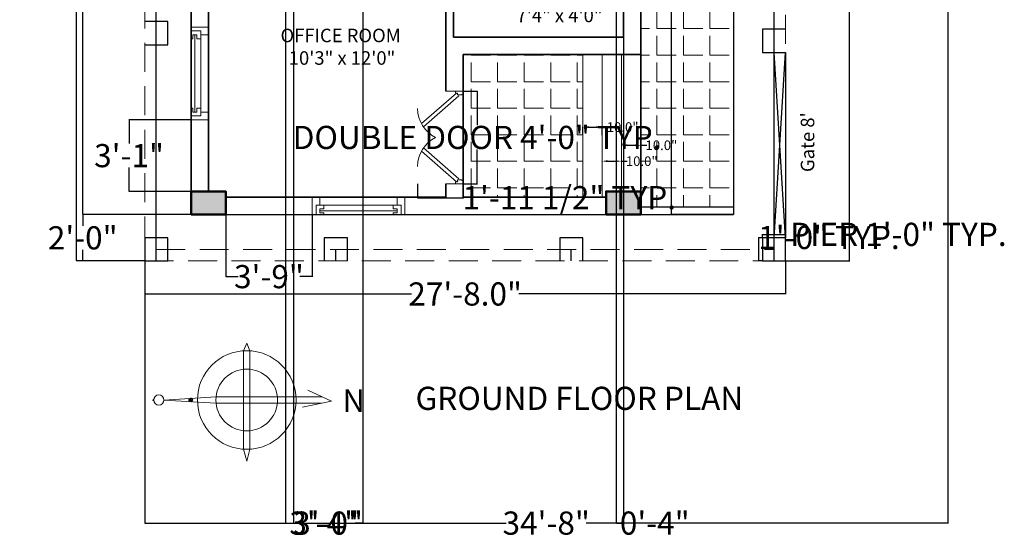
# Model space of a CAD drawing. Units: inches. Extents: x 1063 to 2718, y 423 to 1923.
# Tile 1 of 7: x 1086 to 1596, y 423 to 692. Entities that reach past the tile are written whole.
import ezdxf

# ---------------------------------------------------------------- set-up
doc = ezdxf.new("R2010")
doc.units = ezdxf.units.IN
doc.header["$LTSCALE"] = 6
doc.header["$MEASUREMENT"] = 0
doc.linetypes.add('HIDDEN', pattern=[0.375, 0.25, -0.125])
for name, color, linetype, lineweight in [('A-ANNO-DIMS', 2, 'Continuous', 18), ('A-ANNO-SYMB', 4, 'Continuous', 18), ('A-ANNO-TEXT', 7, 'Continuous', 18), ('A-ANNO-TITL', 7, 'Continuous', 35), ('A-AREA-IDEN', 7, 'Continuous', 18), ('A-COLS', 7, 'Continuous', 50), ('A-COLS-PATT', 252, 'Continuous', 13), ('A-DOOR', 2, 'Continuous', 18), ('A-FLOR', 7, 'Continuous', 25), ('A-FLOR-PATT', 9, 'Continuous', 13), ('A-FLOR-STRS', 7, 'Continuous', 18), ('A-GLAZ', 4, 'Continuous', 18), ('A-WALL', 7, 'Continuous', 35), ('C-GATE', 7, 'Continuous', 25), ('C-PROP', 7, 'Continuous', 25), ('C-PROP-HIDN', 7, 'HIDDEN', 18)]:
    doc.layers.add(name, color=color, linetype=linetype, lineweight=lineweight)
doc.styles.get("Standard").update_dxf_attribs({"font": 'arial.ttf'})
doc.dimstyles.get("Standard").update_dxf_attribs({"dimtxt": 12, "dimasz": 0.18, "dimexe": 0.18, "dimexo": 0.0625, "dimgap": 0.09, "dimtad": 0, "dimtih": 1, "dimtoh": 1, "dimdec": 1, "dimzin": 0, "dimdsep": 46, "dimlunit": 3, "dimtxsty": 'Standard', "dimcen": 0.09, "dimadec": 0, "dimazin": 0, "dimtfac": 1, "dimtdec": 1, "dimtofl": 0, "dimtmove": 0, "dimatfit": 3, "dimfxl": 1, "dimtolj": 1, "dimtzin": 0, "dimarcsym": 0})

# ---------------------------------------------------------------- blocks, each defined once
blk = doc.blocks.new('*D1')
at = {"layer": 'A-ANNO-DIMS', "color": 0, "lineweight": -2, "ltscale": 6, "transparency": 16777216}
for p, q in [((1150.86, 1085.12), (1115.44, 1085.12)), ((1115.62, 1084.94), (1115.62, 832.34)), ((1115.62, 567.3), (1115.62, 819.9)), ((1150.86, 567.12), (1115.44, 567.12))]:
    blk.add_line(p, q, dxfattribs=at)
at = {"layer": 'A-ANNO-DIMS', "color": 0, "ltscale": 6, "transparency": 16777216}
for points in [[(1115.59, 1084.94), (1115.65, 1084.94), (1115.62, 1085.12)], [(1115.59, 567.3), (1115.65, 567.3), (1115.62, 567.12)]]:
    blk.add_solid(points, dxfattribs=at)
at = {"layer": 'Defpoints', "color": 0, "ltscale": 6, "transparency": 16777216}
for p in [(1115.62, 1085.12), (1150.93, 1085.12), (1150.93, 567.12)]:
    blk.add_point(p, dxfattribs=at)
at = {"layer": 'A-ANNO-DIMS', "color": 0, "ltscale": 6, "transparency": 16777216, "insert": (1115.62, 826.12), "char_height": 12, "attachment_point": 5}
blk.add_mtext('\\A1;43\'-2.0"', dxfattribs=at)
blk = doc.blocks.new('*D2')
at = {"layer": 'A-ANNO-DIMS', "color": 0, "lineweight": -2, "ltscale": 6, "transparency": 16777216}
for p, q in [((1150.93, 567.06), (1150.93, 549.86)), ((1482.93, 567.06), (1482.93, 549.86)), ((1151.11, 550.04), (1289.13, 550.04)), ((1482.75, 550.04), (1344.72, 550.04))]:
    blk.add_line(p, q, dxfattribs=at)
at = {"layer": 'A-ANNO-DIMS', "color": 0, "ltscale": 6, "transparency": 16777216}
for points in [[(1151.11, 550.07), (1151.11, 550.01), (1150.93, 550.04)], [(1482.75, 550.07), (1482.75, 550.01), (1482.93, 550.04)]]:
    blk.add_solid(points, dxfattribs=at)
at = {"layer": 'Defpoints', "color": 0, "ltscale": 6, "transparency": 16777216}
for p in [(1150.93, 567.12), (1482.93, 567.12), (1482.93, 550.04)]:
    blk.add_point(p, dxfattribs=at)
at = {"layer": 'A-ANNO-DIMS', "color": 0, "ltscale": 6, "transparency": 16777216, "insert": (1316.93, 550.04), "char_height": 12, "attachment_point": 5}
blk.add_mtext('\\A1;27\'-8.0"', dxfattribs=at)
blk = doc.blocks.new('*D3')
at = {"layer": 'A-ANNO-DIMS', "color": 0, "lineweight": -2, "ltscale": 6, "transparency": 16777216}
for p, q in [((1482.99, 951.12), (1516.18, 951.12)), ((1516, 950.94), (1516, 765.34)), ((1516, 567.3), (1516, 752.9)), ((1482.99, 567.12), (1516.18, 567.12))]:
    blk.add_line(p, q, dxfattribs=at)
at = {"layer": 'A-ANNO-DIMS', "color": 0, "ltscale": 6, "transparency": 16777216}
for points in [[(1515.97, 950.94), (1516.03, 950.94), (1516, 951.12)], [(1515.97, 567.3), (1516.03, 567.3), (1516, 567.12)]]:
    blk.add_solid(points, dxfattribs=at)
at = {"layer": 'Defpoints', "color": 0, "ltscale": 6, "transparency": 16777216}
for p in [(1482.93, 951.12), (1516, 951.12), (1482.93, 567.12)]:
    blk.add_point(p, dxfattribs=at)
at = {"layer": 'A-ANNO-DIMS', "color": 0, "ltscale": 6, "transparency": 16777216, "insert": (1516, 759.12), "char_height": 12, "attachment_point": 5}
blk.add_mtext("\\A1;32'", dxfattribs=at)
blk = doc.blocks.new('*D11')
at = {"layer": 'A-ANNO-DIMS', "color": 0, "lineweight": -2, "ltscale": 6, "transparency": 16777216}
for p, q in [((1377.93, 632.3), (1377.93, 636.66)), ((1380.93, 636.48), (1384.93, 636.48)), ((1387.93, 632.3), (1387.93, 636.66)), ((1387.93, 636.48), (1390.93, 636.48))]:
    blk.add_line(p, q, dxfattribs=at)
at = {"layer": 'A-ANNO-DIMS', "color": 0, "ltscale": 6, "transparency": 16777216}
for points in [[(1380.93, 636.98), (1380.93, 635.98), (1377.93, 636.48)], [(1384.93, 636.98), (1384.93, 635.98), (1387.93, 636.48)]]:
    blk.add_solid(points, dxfattribs=at)
at = {"layer": 'Defpoints', "color": 0, "ltscale": 6, "transparency": 16777216}
for p in [(1387.93, 636.48), (1377.93, 632.24), (1387.93, 632.24)]:
    blk.add_point(p, dxfattribs=at)
at = {"layer": 'A-ANNO-DIMS', "color": 0, "ltscale": 6, "transparency": 16777216, "insert": (1398.51, 636.48), "char_height": 5, "attachment_point": 5}
blk.add_mtext('\\A1;10.0"', dxfattribs=at)
blk = doc.blocks.new('*D12')
at = {"layer": 'A-ANNO-DIMS', "color": 0, "lineweight": -2, "ltscale": 6, "transparency": 16777216}
for p, q in [((1387.84, 618.89), (1387.84, 619.01)), ((1390.84, 618.83), (1394.84, 618.83)), ((1397.84, 618.89), (1397.84, 619.01)), ((1397.84, 618.83), (1400.84, 618.83))]:
    blk.add_line(p, q, dxfattribs=at)
at = {"layer": 'A-ANNO-DIMS', "color": 0, "ltscale": 6, "transparency": 16777216}
for points in [[(1390.84, 619.33), (1390.84, 618.33), (1387.84, 618.83)], [(1394.84, 619.33), (1394.84, 618.33), (1397.84, 618.83)]]:
    blk.add_solid(points, dxfattribs=at)
at = {"layer": 'Defpoints', "color": 0, "ltscale": 6, "transparency": 16777216}
for p in [(1387.84, 618.83), (1397.84, 618.83), (1397.84, 618.83)]:
    blk.add_point(p, dxfattribs=at)
at = {"layer": 'A-ANNO-DIMS', "color": 0, "ltscale": 6, "transparency": 16777216, "insert": (1408.42, 618.83), "char_height": 5, "attachment_point": 5}
blk.add_mtext('\\A1;10.0"', dxfattribs=at)
blk = doc.blocks.new('*D13')
at = {"layer": 'A-ANNO-DIMS', "color": 0, "lineweight": -2, "ltscale": 6, "transparency": 16777216}
for p, q in [((1398.02, 628.06), (1398.02, 626.89)), ((1408.02, 628.06), (1408.02, 626.89)), ((1401.02, 627.07), (1405.02, 627.07)), ((1408.02, 627.07), (1411.02, 627.07))]:
    blk.add_line(p, q, dxfattribs=at)
at = {"layer": 'A-ANNO-DIMS', "color": 0, "ltscale": 6, "transparency": 16777216}
for points in [[(1401.02, 627.57), (1401.02, 626.57), (1398.02, 627.07)], [(1405.02, 627.57), (1405.02, 626.57), (1408.02, 627.07)]]:
    blk.add_solid(points, dxfattribs=at)
at = {"layer": 'Defpoints', "color": 0, "ltscale": 6, "transparency": 16777216}
for p in [(1398.02, 628.12), (1408.02, 628.12), (1408.02, 627.07)]:
    blk.add_point(p, dxfattribs=at)
at = {"layer": 'A-ANNO-DIMS', "color": 0, "ltscale": 6, "transparency": 16777216, "insert": (1418.6, 627.07), "char_height": 5, "attachment_point": 5}
blk.add_mtext('\\A1;10.0"', dxfattribs=at)
blk = doc.blocks.new('WIN-48-SLIDING')
at = {"ltscale": 6}
for p, q in [((0, 9), (4, 9)), ((4, 9), (4, 5)), ((48, 9), (44, 9)), ((44, 9), (44, 5)), ((4, 5), (2, 5)), ((2, 5), (2, 0)), ((4, 5), (44, 5)), ((4, 5), (6, 5)), ((6, 3), (4, 3)), ((4, 3), (4, 1)), ((4, 2), (44, 2)), ((4, 1), (6, 1)), ((6, 5), (6, 3)), ((6, 1), (6, 0)), ((44, 5), (42, 5)), ((42, 5), (42, 3)), ((42, 3), (44, 3)), ((44, 1), (42, 1)), ((42, 1), (42, 0)), ((44, 5), (46, 5)), ((44, 3), (44, 1)), ((46, 5), (46, 0)), ((48, 0), (0, 0)), ((2, 0), (46, 0))]:
    blk.add_line(p, q, dxfattribs=at)
blk.add_lwpolyline([(48, 0), (48, 9), (0, 9), (0, 0)], dxfattribs=at)
blk = doc.blocks.new('DOOR-48-DOUBLE-SWING')
at = {"ltscale": 6}
for p, q in [((20.22, 47), (2.07, 31.16)), ((19.72, 48), (19.72, 47)), ((19.72, 47), (20.72, 47)), ((20.72, 47), (20.72, 46)), ((20.72, 46), (23.03, 46)), ((23.19, 46.24), (23.03, 46.24)), ((23.03, 46.24), (23.03, 46)), ((23.72, 46.54), (23.39, 46.54)), ((23.39, 46.54), (23.39, 46.44)), ((21.53, 45.49), (3.14, 29.43)), ((20.22, 1), (2.07, 16.84)), ((21.53, 2.51), (3.14, 18.57)), ((19.72, 0), (19.72, 1)), ((19.72, 1), (20.72, 1)), ((20.72, 1), (20.72, 2)), ((20.72, 2), (23.03, 2)), ((23.03, 1.76), (23.03, 2)), ((23.19, 1.76), (23.03, 1.76)), ((23.39, 1.46), (23.39, 1.56)), ((23.72, 1.46), (23.39, 1.46))]:
    blk.add_line(p, q, dxfattribs=at)
for p, q in [((14.72, 48), (23.72, 48)), ((23.72, 0), (14.72, 0))]:
    blk.add_line(p, q)
for centre, radius, start, end in [((23.19, 46.44), 0.2, 270, 0), ((17.26, 39.37), 17.27, 181.2158, 242.8966), ((17.26, 8.63), 17.27, 117.1034, 178.7842), ((23.19, 1.56), 0.2, 0, 90)]:
    blk.add_arc(centre, radius, start, end, dxfattribs=at)
blk = doc.blocks.new('COLUMN-18X12')
blk.add_lwpolyline([(0, 0), (18, 0), (18, 12), (0, 12)], close=True)
blk = doc.blocks.new('PIER-12X12')
blk.add_lwpolyline([(0, 0), (12, 0), (12, 12), (0, 12)], close=True)
blk = doc.blocks.new('PIER-12X12-INLINE')
blk.add_lwpolyline([(0, 0), (12, 0), (12, 12), (0, 12)])
blk = doc.blocks.new('*D30')
at = {"layer": 'A-ANNO-DIMS', "color": 0, "lineweight": -2, "ltscale": 6, "transparency": 16777216}
for p, q in [((1470.93, 579.18), (1470.93, 581.1)), ((1471.11, 580.92), (1482.75, 580.92)), ((1482.93, 579.18), (1482.93, 581.1)), ((1482.93, 580.92), (1483.11, 580.92))]:
    blk.add_line(p, q, dxfattribs=at)
at = {"layer": 'A-ANNO-DIMS', "color": 0, "ltscale": 6, "transparency": 16777216}
for points in [[(1471.11, 580.95), (1471.11, 580.89), (1470.93, 580.92)], [(1482.75, 580.95), (1482.75, 580.89), (1482.93, 580.92)]]:
    blk.add_solid(points, dxfattribs=at)
at = {"layer": 'Defpoints', "color": 0, "ltscale": 6, "transparency": 16777216}
for p in [(1470.93, 579.12), (1482.93, 580.92), (1482.93, 579.12)]:
    blk.add_point(p, dxfattribs=at)
at = {"layer": 'A-ANNO-DIMS', "color": 0, "ltscale": 6, "transparency": 16777216, "insert": (1541.36, 580.92), "char_height": 12, "attachment_point": 5}
blk.add_mtext('\\A1;PIER 1\'-0" TYP.', dxfattribs=at)
blk = doc.blocks.new('*D31')
at = {"layer": 'A-ANNO-DIMS', "color": 0, "lineweight": -2, "ltscale": 6, "transparency": 16777216}
for p, q in [((1470.86, 579.12), (1468.95, 579.12)), ((1469.13, 579.12), (1469.13, 579.3)), ((1469.13, 579.3), (1469.31, 579.3)), ((1469.13, 567.3), (1469.13, 578.94)), ((1470.86, 567.12), (1468.95, 567.12))]:
    blk.add_line(p, q, dxfattribs=at)
at = {"layer": 'A-ANNO-DIMS', "color": 0, "ltscale": 6, "transparency": 16777216}
for points in [[(1469.1, 578.94), (1469.16, 578.94), (1469.13, 579.12)], [(1469.1, 567.3), (1469.16, 567.3), (1469.13, 567.12)]]:
    blk.add_solid(points, dxfattribs=at)
at = {"layer": 'Defpoints', "color": 0, "ltscale": 6, "transparency": 16777216}
for p in [(1469.13, 579.12), (1470.93, 579.12), (1470.93, 567.12)]:
    blk.add_point(p, dxfattribs=at)
at = {"layer": 'A-ANNO-DIMS', "color": 0, "ltscale": 6, "transparency": 16777216, "insert": (1505.4, 579.3), "char_height": 12, "attachment_point": 5}
blk.add_mtext('\\A1;1\'-0" TYP.', dxfattribs=at)
blk = doc.blocks.new('*D40')
at = {"layer": 'A-ANNO-DIMS', "color": 0, "lineweight": -2, "ltscale": 6, "transparency": 16777216}
for p, q in [((1315.99, 655.12), (1323.31, 655.12)), ((1323.13, 654.94), (1323.13, 637.42)), ((1323.13, 607.3), (1323.13, 624.82)), ((1315.99, 607.12), (1323.31, 607.12))]:
    blk.add_line(p, q, dxfattribs=at)
at = {"layer": 'A-ANNO-DIMS', "color": 0, "ltscale": 6, "transparency": 16777216}
for points in [[(1323.1, 654.94), (1323.16, 654.94), (1323.13, 655.12)], [(1323.1, 607.3), (1323.16, 607.3), (1323.13, 607.12)]]:
    blk.add_solid(points, dxfattribs=at)
at = {"layer": 'Defpoints', "color": 0, "ltscale": 6, "transparency": 16777216}
for p in [(1315.93, 655.12), (1323.13, 655.12), (1315.93, 607.12)]:
    blk.add_point(p, dxfattribs=at)
at = {"layer": 'A-ANNO-DIMS', "color": 0, "ltscale": 6, "transparency": 16777216, "insert": (1323.13, 631.12), "char_height": 12, "attachment_point": 5}
blk.add_mtext('\\A1;DOUBLE DOOR 4\'-0" TYP.', dxfattribs=at)
blk = doc.blocks.new('*D41')
at = {"layer": 'A-ANNO-DIMS', "color": 0, "lineweight": -2, "ltscale": 6, "transparency": 16777216}
for p, q in [((1292.21, 607.06), (1292.21, 599.74)), ((1315.93, 607.06), (1315.93, 599.74)), ((1292.39, 599.92), (1315.75, 599.92)), ((1315.93, 599.92), (1316.11, 599.92))]:
    blk.add_line(p, q, dxfattribs=at)
at = {"layer": 'A-ANNO-DIMS', "color": 0, "ltscale": 6, "transparency": 16777216}
for points in [[(1292.39, 599.95), (1292.39, 599.89), (1292.21, 599.92)], [(1315.75, 599.95), (1315.75, 599.89), (1315.93, 599.92)]]:
    blk.add_solid(points, dxfattribs=at)
at = {"layer": 'Defpoints', "color": 0, "ltscale": 6, "transparency": 16777216}
for p in [(1292.21, 607.12), (1315.93, 607.12), (1315.93, 599.92)]:
    blk.add_point(p, dxfattribs=at)
at = {"layer": 'A-ANNO-DIMS', "color": 0, "ltscale": 6, "transparency": 16777216, "insert": (1370.85, 599.92), "char_height": 12, "attachment_point": 5}
blk.add_mtext('\\A1;1\'-11 1/2" TYP.', dxfattribs=at)
blk = doc.blocks.new('*D45')
at = {"layer": 'A-ANNO-DIMS', "color": 0, "lineweight": -2, "ltscale": 6, "transparency": 16777216}
for p, q in [((1174.86, 1055.12), (1118.65, 1055.12)), ((1118.83, 1054.94), (1118.83, 829.34)), ((1118.83, 591.3), (1118.83, 816.9)), ((1174.86, 591.12), (1118.65, 591.12))]:
    blk.add_line(p, q, dxfattribs=at)
at = {"layer": 'A-ANNO-DIMS', "color": 0, "ltscale": 6, "transparency": 16777216}
for points in [[(1118.8, 1054.94), (1118.86, 1054.94), (1118.83, 1055.12)], [(1118.8, 591.3), (1118.86, 591.3), (1118.83, 591.12)]]:
    blk.add_solid(points, dxfattribs=at)
at = {"layer": 'Defpoints', "color": 0, "ltscale": 6, "transparency": 16777216}
for p in [(1118.83, 1055.12), (1174.93, 1055.12), (1174.93, 591.12)]:
    blk.add_point(p, dxfattribs=at)
at = {"layer": 'A-ANNO-DIMS', "color": 0, "ltscale": 6, "transparency": 16777216, "insert": (1118.83, 823.12), "char_height": 12, "attachment_point": 5}
blk.add_mtext('\\A1;38\'-8"', dxfattribs=at)
blk = doc.blocks.new('*D47')
at = {"layer": 'A-ANNO-DIMS', "color": 0, "lineweight": -2, "ltscale": 6, "transparency": 16777216}
for p, q in [((1174.86, 591.12), (1118.65, 591.12)), ((1118.83, 590.94), (1118.83, 585.34)), ((1118.83, 567.3), (1118.83, 572.9)), ((1150.86, 567.12), (1118.65, 567.12))]:
    blk.add_line(p, q, dxfattribs=at)
at = {"layer": 'A-ANNO-DIMS', "color": 0, "ltscale": 6, "transparency": 16777216}
for points in [[(1118.8, 590.94), (1118.86, 590.94), (1118.83, 591.12)], [(1118.8, 567.3), (1118.86, 567.3), (1118.83, 567.12)]]:
    blk.add_solid(points, dxfattribs=at)
at = {"layer": 'Defpoints', "color": 0, "ltscale": 6, "transparency": 16777216}
for p in [(1118.83, 591.12), (1174.93, 591.12), (1150.93, 567.12)]:
    blk.add_point(p, dxfattribs=at)
at = {"layer": 'A-ANNO-DIMS', "color": 0, "ltscale": 6, "transparency": 16777216, "insert": (1118.83, 579.12), "char_height": 12, "attachment_point": 5}
blk.add_mtext('\\A1;2\'-0"', dxfattribs=at)
blk = doc.blocks.new('*D50')
at = {"layer": 'A-ANNO-DIMS', "color": 0, "lineweight": -2, "ltscale": 6, "transparency": 16777216}
for p, q in [((1566.93, 731.06), (1566.93, 431.18)), ((1150.93, 567.06), (1150.93, 431.18)), ((1151.11, 431.36), (1338.23, 431.36)), ((1566.75, 431.36), (1379.62, 431.36))]:
    blk.add_line(p, q, dxfattribs=at)
at = {"layer": 'A-ANNO-DIMS', "color": 0, "ltscale": 6, "transparency": 16777216}
for points in [[(1151.11, 431.39), (1151.11, 431.33), (1150.93, 431.36)], [(1566.75, 431.39), (1566.75, 431.33), (1566.93, 431.36)]]:
    blk.add_solid(points, dxfattribs=at)
at = {"layer": 'Defpoints', "color": 0, "ltscale": 6, "transparency": 16777216}
for p in [(1566.93, 731.12), (1150.93, 567.12), (1566.93, 431.36)]:
    blk.add_point(p, dxfattribs=at)
at = {"layer": 'A-ANNO-DIMS', "color": 0, "ltscale": 6, "transparency": 16777216, "insert": (1358.93, 431.36), "char_height": 12, "attachment_point": 5}
blk.add_mtext('\\A1;34\'-8"', dxfattribs=at)
blk = doc.blocks.new('*D52')
at = {"layer": 'A-ANNO-DIMS', "color": 0, "lineweight": -2, "ltscale": 6, "transparency": 16777216}
for p, q in [((1455.86, 910.12), (1423.65, 910.12)), ((1423.83, 909.94), (1423.83, 756.84)), ((1423.83, 591.3), (1423.83, 744.4)), ((1455.86, 591.12), (1423.65, 591.12))]:
    blk.add_line(p, q, dxfattribs=at)
at = {"layer": 'A-ANNO-DIMS', "color": 0, "ltscale": 6, "transparency": 16777216}
for points in [[(1423.8, 909.94), (1423.86, 909.94), (1423.83, 910.12)], [(1423.8, 591.3), (1423.86, 591.3), (1423.83, 591.12)]]:
    blk.add_solid(points, dxfattribs=at)
at = {"layer": 'Defpoints', "color": 0, "ltscale": 6, "transparency": 16777216}
for p in [(1423.83, 910.12), (1455.93, 910.12), (1455.93, 591.12)]:
    blk.add_point(p, dxfattribs=at)
at = {"layer": 'A-ANNO-DIMS', "color": 0, "ltscale": 6, "transparency": 16777216, "insert": (1423.83, 750.62), "char_height": 12, "attachment_point": 5}
blk.add_mtext('\\A1;26\'-7"', dxfattribs=at)
blk = doc.blocks.new('*D55')
at = {"layer": 'A-ANNO-DIMS', "color": 0, "lineweight": -2, "ltscale": 6, "transparency": 16777216}
for p, q in [((1227.93, 860.06), (1227.93, 431.18)), ((1263.93, 860.06), (1263.93, 431.18)), ((1228.11, 431.36), (1229.89, 431.36)), ((1263.75, 431.36), (1261.96, 431.36))]:
    blk.add_line(p, q, dxfattribs=at)
at = {"layer": 'A-ANNO-DIMS', "color": 0, "ltscale": 6, "transparency": 16777216}
for points in [[(1228.11, 431.39), (1228.11, 431.33), (1227.93, 431.36)], [(1263.75, 431.39), (1263.75, 431.33), (1263.93, 431.36)]]:
    blk.add_solid(points, dxfattribs=at)
at = {"layer": 'Defpoints', "color": 0, "ltscale": 6, "transparency": 16777216}
for p in [(1227.93, 860.12), (1263.93, 860.12), (1263.93, 431.36)]:
    blk.add_point(p, dxfattribs=at)
at = {"layer": 'A-ANNO-DIMS', "color": 0, "ltscale": 6, "transparency": 16777216, "insert": (1245.93, 431.36), "char_height": 12, "attachment_point": 5}
blk.add_mtext('\\A1;3\'-0"', dxfattribs=at)
blk = doc.blocks.new('*D58')
at = {"layer": 'A-ANNO-DIMS', "color": 0, "lineweight": -2, "ltscale": 6, "transparency": 16777216}
for p, q in [((1223.93, 748.06), (1223.93, 431.18)), ((1263.93, 748.06), (1263.93, 431.18)), ((1224.11, 431.36), (1227.89, 431.36)), ((1263.75, 431.36), (1259.96, 431.36))]:
    blk.add_line(p, q, dxfattribs=at)
at = {"layer": 'A-ANNO-DIMS', "color": 0, "ltscale": 6, "transparency": 16777216}
for points in [[(1224.11, 431.39), (1224.11, 431.33), (1223.93, 431.36)], [(1263.75, 431.39), (1263.75, 431.33), (1263.93, 431.36)]]:
    blk.add_solid(points, dxfattribs=at)
at = {"layer": 'Defpoints', "color": 0, "ltscale": 6, "transparency": 16777216}
for p in [(1223.93, 748.12), (1263.93, 748.12), (1263.93, 431.36)]:
    blk.add_point(p, dxfattribs=at)
at = {"layer": 'A-ANNO-DIMS', "color": 0, "ltscale": 6, "transparency": 16777216, "insert": (1243.93, 431.36), "char_height": 12, "attachment_point": 5}
blk.add_mtext('\\A1;3\'-4"', dxfattribs=at)
blk = doc.blocks.new('*D65')
at = {"layer": 'A-ANNO-DIMS', "color": 0, "lineweight": -2, "ltscale": 6, "transparency": 16777216}
for p, q in [((1395.08, 961.04), (1395.08, 431.18)), ((1398.93, 954.06), (1398.93, 431.18)), ((1395.26, 431.36), (1398.75, 431.36)), ((1398.93, 431.36), (1399.11, 431.36))]:
    blk.add_line(p, q, dxfattribs=at)
at = {"layer": 'A-ANNO-DIMS', "color": 0, "ltscale": 6, "transparency": 16777216}
for points in [[(1395.26, 431.39), (1395.26, 431.33), (1395.08, 431.36)], [(1398.75, 431.39), (1398.75, 431.33), (1398.93, 431.36)]]:
    blk.add_solid(points, dxfattribs=at)
at = {"layer": 'Defpoints', "color": 0, "ltscale": 6, "transparency": 16777216}
for p in [(1395.08, 961.11), (1398.93, 954.12), (1398.93, 431.36)]:
    blk.add_point(p, dxfattribs=at)
at = {"layer": 'A-ANNO-DIMS', "color": 0, "ltscale": 6, "transparency": 16777216, "insert": (1415.15, 431.36), "char_height": 12, "attachment_point": 5}
blk.add_mtext('\\A1;0\'-4"', dxfattribs=at)
blk = doc.blocks.new('*D68')
at = {"layer": 'A-ANNO-DIMS', "color": 0, "lineweight": -2, "ltscale": 6, "transparency": 16777216}
for p, q in [((1174.86, 640.28), (1142.65, 640.28)), ((1142.83, 640.1), (1142.83, 627.92)), ((1142.83, 603.3), (1142.83, 615.48)), ((1174.86, 603.12), (1142.65, 603.12))]:
    blk.add_line(p, q, dxfattribs=at)
at = {"layer": 'A-ANNO-DIMS', "color": 0, "ltscale": 6, "transparency": 16777216}
for points in [[(1142.8, 640.1), (1142.86, 640.1), (1142.83, 640.28)], [(1142.8, 603.3), (1142.86, 603.3), (1142.83, 603.12)]]:
    blk.add_solid(points, dxfattribs=at)
at = {"layer": 'Defpoints', "color": 0, "ltscale": 6, "transparency": 16777216}
for p in [(1142.83, 640.28), (1174.93, 640.28), (1174.93, 603.12)]:
    blk.add_point(p, dxfattribs=at)
at = {"layer": 'A-ANNO-DIMS', "color": 0, "ltscale": 6, "transparency": 16777216, "insert": (1142.83, 621.7), "char_height": 12, "attachment_point": 5}
blk.add_mtext('\\A1;3\'-1"', dxfattribs=at)
blk = doc.blocks.new('*D69')
at = {"layer": 'A-ANNO-DIMS', "color": 0, "lineweight": -2, "ltscale": 6, "transparency": 16777216}
for p, q in [((1192.93, 591.06), (1192.93, 558.84)), ((1237.71, 591.06), (1237.71, 558.84)), ((1193.11, 559.02), (1199.28, 559.02)), ((1237.53, 559.02), (1231.35, 559.02))]:
    blk.add_line(p, q, dxfattribs=at)
at = {"layer": 'A-ANNO-DIMS', "color": 0, "ltscale": 6, "transparency": 16777216}
for points in [[(1193.11, 559.05), (1193.11, 558.99), (1192.93, 559.02)], [(1237.53, 559.05), (1237.53, 558.99), (1237.71, 559.02)]]:
    blk.add_solid(points, dxfattribs=at)
at = {"layer": 'Defpoints', "color": 0, "ltscale": 6, "transparency": 16777216}
for p in [(1192.93, 591.12), (1237.71, 591.12), (1192.93, 559.02)]:
    blk.add_point(p, dxfattribs=at)
at = {"layer": 'A-ANNO-DIMS', "color": 0, "ltscale": 6, "transparency": 16777216, "insert": (1215.32, 559.02), "char_height": 12, "attachment_point": 5}
blk.add_mtext('\\A1;3\'-9"', dxfattribs=at)

msp = doc.modelspace()

# ---------------------------------------------------------------- hatches: boundary and pattern name
at = {"layer": 'A-COLS-PATT', "ltscale": 6}
h = msp.add_hatch(color=256, dxfattribs=at)
h.dxf.hatch_style = 1
h.paths.add_polyline_path([(1192.93, 603.12), (1174.93, 603.12), (1174.93, 591.12), (1192.93, 591.12)])
h.paths.add_polyline_path([(1407.93, 603.12), (1389.93, 603.12), (1389.93, 591.12), (1407.93, 591.12)])
h.paths.add_polyline_path([(1192.93, 756.12), (1174.93, 756.12), (1174.93, 744.12), (1192.93, 744.12)])
h.paths.add_polyline_path([(1407.93, 761.11), (1389.93, 761.11), (1389.93, 749.11), (1407.93, 749.11)])
h.paths.add_polyline_path([(1455.93, 761.11), (1437.93, 761.11), (1437.93, 749.11), (1455.93, 749.11)])
h.paths.add_polyline_path([(1455.93, 910.12), (1437.93, 910.12), (1437.93, 898.12), (1455.93, 898.12)])
h.paths.add_polyline_path([(1407.93, 910.12), (1389.93, 910.12), (1389.93, 898.12), (1407.93, 898.12)])
h.paths.add_polyline_path([(1192.93, 910.12), (1174.93, 910.12), (1174.93, 898.12), (1192.93, 898.12)])
h.paths.add_polyline_path([(1192.93, 1055.12), (1174.93, 1055.12), (1174.93, 1043.12), (1192.93, 1043.12)])
h.paths.add_polyline_path([(1407.93, 1055.12), (1389.93, 1055.12), (1389.93, 1043.12), (1407.93, 1043.12)])
at = {"layer": 'A-FLOR-PATT', "ltscale": 6}
h = msp.add_hatch(dxfattribs=at)
h.set_pattern_fill('ANGLE', color=256, scale=50)
h.set_pattern_definition([(0, (0, 0), (0, 13.75), [10, -3.75]), (90, (0, 0), (-13.75, 8e-16), [10, -3.75])])
h.paths.add_polyline_path([(1455.93, 749.11), (1437.93, 749.11), (1437.93, 761.11), (1455.93, 761.11), (1455.93, 868.12), (1407.93, 868.12), (1407.93, 595.12), (1455.93, 595.12)])
h.paths.add_polyline_path([(1377.93, 674.12), (1315.93, 674.12), (1315.93, 600.12), (1377.93, 600.12)])

# ---------------------------------------------------------------- linework, layer by layer
at = {"layer": 'A-ANNO-SYMB', "ltscale": 6}
for p, q in [((1202.12, 520.61), (1203.8, 524.59)), ((1202.12, 520.67), (1202.12, 469.58)), ((1203.8, 524.59), (1205.48, 520.67)), ((1205.48, 520.67), (1205.48, 469.58)), ((1247.67, 494.56), (1235.44, 500.16)), ((1187.91, 496.8), (1160.88, 495.12)), ((1187.83, 493.44), (1160.88, 495.12)), ((1187.83, 496.8), (1242.77, 496.8)), ((1187.83, 493.44), (1242.38, 493.44)), ((1247.67, 494.56), (1232.61, 491.39)), ((1202.12, 469.63), (1203.8, 463.46)), ((1203.8, 463.46), (1205.48, 469.63))]:
    msp.add_line(p, q, dxfattribs=at)
for points in [[(1174.63, 496.1), (1173.86, 495.63), (1173.83, 494.83), (1174.51, 494.28)], [(1174.93, 496.06), (1174.16, 495.59), (1174.13, 494.79), (1174.81, 494.24)], [(1175.25, 496.06), (1174.47, 495.59), (1174.45, 494.79), (1175.12, 494.24)], [(1175.55, 496.03), (1174.77, 495.56), (1174.75, 494.76), (1175.43, 494.22)], [(1175.83, 495.57), (1175.3, 495.25), (1175.29, 495.01), (1175.76, 494.63)], [(1175.9, 495.46), (1175.43, 495.18), (1175.43, 495.07), (1175.84, 494.73)]]:
    msp.add_lwpolyline(points, dxfattribs=at)
for centre, radius in [((1203.8, 495.12), 25.55), ((1203.8, 495.12), 15.97), ((1158.24, 495.12), 2.64)]:
    msp.add_circle(centre, radius, dxfattribs=at)
msp.add_arc((1155.6, 495.12), 0.372, 85.9568, 274.0432, dxfattribs=at)
at = {"layer": 'A-FLOR'}
for p, q in [((1455.93, 898.12), (1455.93, 591.12)), ((1407.93, 595.12), (1455.93, 595.12))]:
    msp.add_line(p, q, dxfattribs=at)
at = {"layer": 'A-FLOR', "ltscale": 6}
msp.add_line((1174.93, 591.12), (1455.93, 591.12), dxfattribs=at)
at = {"layer": 'A-FLOR-STRS'}
for p, q in [((1377.93, 674.12), (1377.93, 600.12)), ((1387.93, 674.12), (1387.93, 600.12)), ((1397.93, 674.12), (1397.93, 603.12))]:
    msp.add_line(p, q, dxfattribs=at)
at = {"layer": 'A-WALL', "ltscale": 6}
for p, q in [((1174.93, 1055.12), (1174.93, 591.12)), ((1407.93, 1055.12), (1407.93, 591.12)), ((1183.93, 744.12), (1183.93, 603.12)), ((1192.93, 600.12), (1306.93, 600.12))]:
    msp.add_line(p, q, dxfattribs=at)
at = {"layer": 'A-WALL'}
for p, q in [((1306.93, 744.12), (1306.93, 655.12)), ((1310.93, 731.12), (1310.93, 683.12)), ((1398.93, 731.12), (1398.93, 683.12)), ((1310.93, 683.12), (1398.93, 683.12)), ((1315.93, 674.12), (1407.93, 674.12)), ((1315.93, 674.12), (1315.93, 600.12)), ((1306.93, 607.12), (1306.93, 600.12)), ((1315.93, 600.12), (1389.93, 600.12))]:
    msp.add_line(p, q, dxfattribs=at)
at = {"layer": 'C-GATE', "ltscale": 6}
for p, q in [((1476.93, 579.12), (1482.93, 675.12)), ((1482.93, 579.12), (1476.93, 675.12)), ((1482.93, 675.12), (1482.93, 579.12))]:
    msp.add_line(p, q, dxfattribs=at)
at = {"layer": 'C-PROP'}
for p, q in [((1156.93, 567.12), (1156.93, 1079.12)), ((1476.93, 567.12), (1476.93, 945.12)), ((1249.93, 567.12), (1249.93, 573.12)), ((1371.93, 567.12), (1371.93, 573.12))]:
    msp.add_line(p, q, dxfattribs=at)
at = {"layer": 'C-PROP-HIDN', "ltscale": 10}
for p, q in [((1150.93, 1085.12), (1150.93, 567.12)), ((1482.93, 567.12), (1482.93, 951.12)), ((1156.93, 573.12), (1476.93, 573.12)), ((1150.93, 567.12), (1482.93, 567.12))]:
    msp.add_line(p, q, dxfattribs=at)

# ---------------------------------------------------------------- block references
at = {"layer": 'A-COLS'}
for p in [(1174.93, 591.12), (1389.93, 591.12)]:
    msp.add_blockref('COLUMN-18X12', p, dxfattribs=at)
at = {"layer": 'A-DOOR'}
msp.add_blockref('DOOR-48-DOUBLE-SWING', (1292.21, 607.12), dxfattribs=at)
at = {"layer": 'A-GLAZ', "rotation": 269.9999999999983}
msp.add_blockref('WIN-48-SLIDING', (1174.93, 688.28), dxfattribs=at)
at = {"layer": 'A-GLAZ'}
msp.add_blockref('WIN-48-SLIDING', (1237.71, 591.12), dxfattribs=at)
at = {"layer": 'C-PROP'}
for name, p in [('PIER-12X12-INLINE', (1150.93, 679.12)), ('PIER-12X12', (1150.93, 567.12)), ('PIER-12X12', (1470.93, 567.12))]:
    msp.add_blockref(name, p, dxfattribs=at)
for p, rotation in [((1482.93, 687.12), 180), ((1255.93, 567.12), 90), ((1377.93, 567.12), 90)]:
    msp.add_blockref('PIER-12X12-INLINE', p, dxfattribs=dict(at, rotation=rotation))

# ---------------------------------------------------------------- texts
at = {"layer": 'A-ANNO-SYMB', "ltscale": 6, "insert": (1253.41, 500.65), "char_height": 11.75, "attachment_point": 1}
msp.add_mtext_dynamic_manual_height_columns('N', width=294.1516, gutter_width=1.68, heights=[0], dxfattribs=at)
at = {"layer": 'A-ANNO-TEXT', "ltscale": 6, "insert": (1490.79, 613.2), "char_height": 7, "attachment_point": 1, "rotation": 90}
msp.add_mtext_dynamic_manual_height_columns("Gate 8'", width=175.2385, gutter_width=1, heights=[0], dxfattribs=at)
at = {"layer": 'A-ANNO-TITL', "ltscale": 6, "insert": (1291.23, 501.98), "char_height": 12, "attachment_point": 1}
msp.add_mtext_dynamic_manual_height_columns('GROUND FLOOR PLAN', width=301.7959, gutter_width=1, heights=[0], dxfattribs=at)
at = {"layer": 'A-AREA-IDEN', "ltscale": 6, "char_height": 7, "attachment_point": 1}
for s, insert in [(' TOILET\\P7\'4" x 4\'0"', (1343.51, 709.48)), ('OFFICE ROOM\\P  10\'3" x 12\'0"', (1221.29, 687.44))]:
    msp.add_mtext_dynamic_manual_height_columns(s, width=175.2385, gutter_width=1, heights=[0], dxfattribs=dict(at, insert=insert))

# ---------------------------------------------------------------- dimensions: what is measured, and where the dimension line sits
at = {"layer": 'A-ANNO-DIMS', "ltscale": 6}
for base, p1, p2, angle, override, picture, middle in [((1115.62, 1085.12), (1150.93, 567.12), (1150.93, 1085.12), 90, {"dimclrd": 0, "dimclre": 0, "dimclrt": 0}, '*D1', (1115.62, 826.12)), ((1118.83, 1055.12), (1174.93, 591.12), (1174.93, 1055.12), 90, {"dimdec": 1, "dimlfac": 1, "dimrnd": 0, "dimzin": 1, "dimdsep": 46, "dimlunit": 4, "dimfrac": 2}, '*D45', (1118.83, 823.12)), ((1516, 951.12), (1482.93, 567.12), (1482.93, 951.12), 90, {"dimclrd": 0, "dimclre": 0, "dimclrt": 0}, '*D3', (1516, 759.12)), ((1423.83, 910.12), (1455.93, 591.12), (1455.93, 910.12), 90, {"dimdec": 1, "dimlfac": 1, "dimrnd": 0, "dimzin": 1, "dimdsep": 46, "dimlunit": 4, "dimfrac": 2}, '*D52', (1423.83, 750.62)), ((1142.83, 640.28), (1174.93, 603.12), (1174.93, 640.28), 90, {"dimdec": 1, "dimlfac": 1, "dimrnd": 0, "dimzin": 1, "dimdsep": 46, "dimlunit": 4, "dimfrac": 2}, '*D68', (1142.83, 621.7)), ((1118.83, 591.12), (1150.93, 567.12), (1174.93, 591.12), 90, {"dimdec": 1, "dimlfac": 1, "dimrnd": 0, "dimzin": 1, "dimdsep": 46, "dimlunit": 4, "dimfrac": 2}, '*D47', (1118.83, 579.12)), ((1192.93, 559.02), (1237.71, 591.12), (1192.93, 591.12), 180, {"dimdec": 1, "dimlfac": 1, "dimrnd": 0, "dimzin": 1, "dimdsep": 46, "dimlunit": 4, "dimfrac": 2}, '*D69', (1215.32, 559.02))]:
    dim = msp.add_linear_dim(base=base, p1=p1, p2=p2, angle=angle, dimstyle='Standard', override=override, dxfattribs=at)
    dim.commit()
    dim.dimension.update_dxf_attribs({"geometry": picture, "text_midpoint": middle})
for base, p1, p2, override, picture, middle in [((1398.9256, 431.3553), (1395.0779, 961.1073), (1398.9256, 954.1189), {"dimdec": 1, "dimlfac": 1, "dimrnd": 0, "dimzin": 1, "dimdsep": 46, "dimlunit": 4, "dimfrac": 2}, '*D65', (1415.1451, 431.3553)), ((1263.93, 431.36), (1227.93, 860.12), (1263.93, 860.12), {"dimdec": 1, "dimlfac": 1, "dimrnd": 0, "dimzin": 1, "dimdsep": 46, "dimlunit": 4, "dimfrac": 2}, '*D55', (1245.93, 431.36)), ((1263.93, 431.36), (1223.93, 748.12), (1263.93, 748.12), {"dimdec": 1, "dimlfac": 1, "dimrnd": 0, "dimzin": 1, "dimdsep": 46, "dimlunit": 4, "dimfrac": 2}, '*D58', (1243.93, 431.36)), ((1566.93, 431.36), (1150.93, 567.12), (1566.93, 731.12), {"dimdec": 1, "dimlfac": 1, "dimrnd": 0, "dimzin": 1, "dimdsep": 46, "dimlunit": 4, "dimfrac": 2}, '*D50', (1358.93, 431.36)), ((1387.93, 636.48), (1377.93, 632.24), (1387.93, 632.24), {"dimtxt": 5, "dimasz": 3, "dimclrd": 0, "dimclre": 0, "dimclrt": 0}, '*D11', (1398.51, 636.48)), ((1408.02, 627.07), (1398.02, 628.12), (1408.02, 628.12), {"dimtxt": 5, "dimasz": 3, "dimclrd": 0, "dimclre": 0, "dimclrt": 0}, '*D13', (1418.6, 627.07)), ((1397.84, 618.83), (1387.84, 618.83), (1397.84, 618.83), {"dimtxt": 5, "dimasz": 3, "dimclrd": 0, "dimclre": 0, "dimclrt": 0}, '*D12', (1408.42, 618.83)), ((1482.93, 550.04), (1150.93, 567.12), (1482.93, 567.12), {"dimclrd": 0, "dimclre": 0, "dimclrt": 0}, '*D2', (1316.93, 550.04))]:
    dim = msp.add_linear_dim(base=base, p1=p1, p2=p2, dimstyle='Standard', override=override, dxfattribs=at)
    dim.commit()
    dim.dimension.update_dxf_attribs({"geometry": picture, "text_midpoint": middle})
for base, p1, p2, text, picture, middle in [((1323.13, 655.12), (1315.93, 607.12), (1315.93, 655.12), 'DOUBLE DOOR <> TYP.', '*D40', (1323.13, 631.12)), ((1469.13, 579.12), (1470.93, 567.12), (1470.93, 579.12), '<> TYP.', '*D31', (1505.4, 579.3))]:
    dim = msp.add_linear_dim(base=base, p1=p1, p2=p2, angle=90, text=text, dimstyle='Standard', override={"dimdec": 1, "dimlfac": 1, "dimrnd": 0, "dimzin": 1, "dimdsep": 46, "dimlunit": 4, "dimfrac": 2}, dxfattribs=at)
    dim.commit()
    dim.dimension.update_dxf_attribs({"geometry": picture, "text_midpoint": middle})
for base, p1, p2, text, picture, middle in [((1315.93, 599.92), (1292.21, 607.12), (1315.93, 607.12), '<> TYP.', '*D41', (1370.85, 599.92)), ((1482.93, 580.92), (1470.93, 579.12), (1482.93, 579.12), 'PIER <> TYP.', '*D30', (1541.36, 580.92))]:
    dim = msp.add_linear_dim(base=base, p1=p1, p2=p2, text=text, dimstyle='Standard', override={"dimdec": 1, "dimlfac": 1, "dimrnd": 0, "dimzin": 1, "dimdsep": 46, "dimlunit": 4, "dimfrac": 2}, dxfattribs=at)
    dim.commit()
    dim.dimension.update_dxf_attribs({"geometry": picture, "text_midpoint": middle})

doc.saveas('drawing.dxf')
